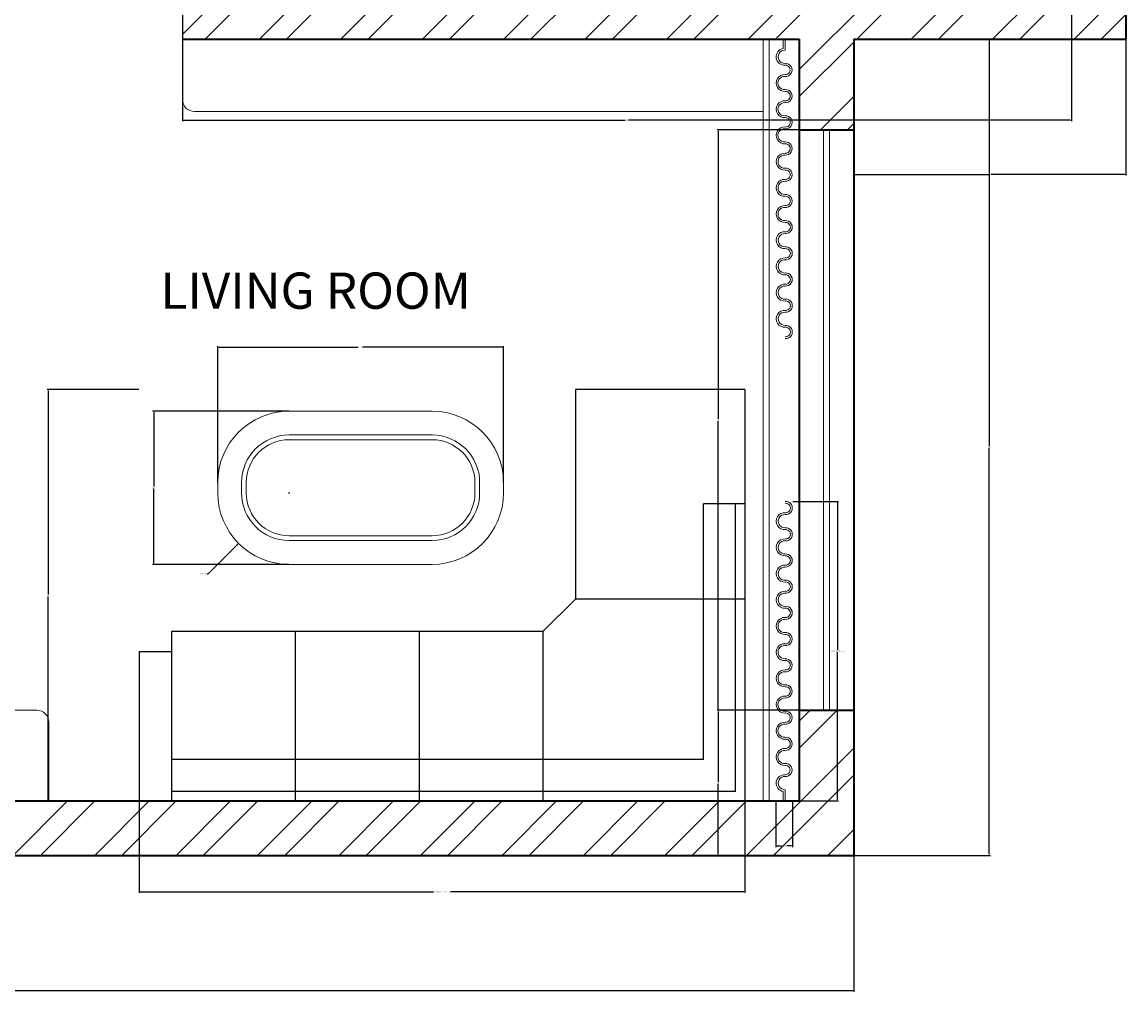
# Model space of a CAD drawing. Units: inches. Extents: x 3449 to 3843, y 1566 to 2054.
# Tile 4 of 8: x 3638 to 3820, y 1566 to 1726. Entities that reach past the tile are written whole.
import ezdxf

# ---------------------------------------------------------------- set-up
doc = ezdxf.new("R2010")
doc.units = ezdxf.units.IN
for name, color, linetype, lineweight in [('A-ANNO-DIMS', 2, 'Continuous', 18), ('A-AREA-IDEN', 7, 'Continuous', 25), ('A-FLOR-CASE', 7, 'Continuous', 20), ('A-FURN-DRAP', 32, 'Continuous', 13), ('A-GLAZ', 5, 'Continuous', 18), ('A-WALL', 7, 'Continuous', 35), ('A-WALL-PATT', 251, 'Continuous', 13), ('furn', 7, 'Continuous', 18)]:
    doc.layers.add(name, color=color, linetype=linetype, lineweight=lineweight)
doc.layers.add('B-FURNITURE', color=22, linetype='Continuous')
doc.styles.get("Standard").update_dxf_attribs({"font": 'arial.ttf'})
doc.dimstyles.get("Standard").update_dxf_attribs({"dimtxt": 0.18, "dimasz": 0.18, "dimexe": 0.18, "dimexo": 0.0625, "dimgap": 0.09, "dimtad": 0, "dimtih": 1, "dimtoh": 1, "dimdec": 4, "dimzin": 0, "dimdsep": 46, "dimtxsty": 'Standard', "dimcen": 0.09, "dimadec": 0, "dimazin": 0, "dimtfac": 1, "dimtdec": 4, "dimtofl": 0, "dimtmove": 0, "dimatfit": 3, "dimfxl": 1, "dimtolj": 1, "dimtzin": 0, "dimarcsym": 0})

# ---------------------------------------------------------------- blocks, each defined once
blk = doc.blocks.new('A$C4399559B')
at = {"layer": 'B-FURNITURE', "ltscale": 100}
for points in [[(-0.712, 0), (0, 0)], [(-0.712, 0), (-0.712, -0.88)], [(0, 0), (0, -0.88)], [(-0.712, -0.48), (-0.5377, -0.48)], [(-0.672, -1.688), (-0.672, -0.48)], [(-0.5377, -1.5537), (-0.5377, -0.48)], [(-0.712, -0.856), (-0.712, -1.728)], [(-0.712, -0.88), (-0.5377, -0.88)], [(-0.5377, -0.88), (0, -0.88)], [(0, -0.856), (0, -0.88)], [(0, -0.88), (0.136, -1.016)], [(0.136, -1.016), (1.696, -1.016)], [(0.136, -1.016), (0.136, -1.728)], [(0.656, -1.016), (0.656, -1.728)], [(1.176, -1.016), (1.176, -1.728)], [(1.696, -1.016), (1.696, -1.728)], [(1.696, -1.1016), (1.832, -1.1016)], [(1.832, -1.1016), (1.832, -1.728)], [(-0.5377, -1.5537), (1.696, -1.5537)], [(-0.672, -1.688), (1.696, -1.688)], [(-0.712, -1.728), (1.832, -1.728)]]:
    blk.add_lwpolyline(points, dxfattribs=at)
blk = doc.blocks.new('DRAPERY-PANEL')
for p, q in [((1.19, 47.95), (1.19, 49.52)), ((1.5, 47.66), (1.5, 49.52))]:
    blk.add_line(p, q)
for centre, radius, start, end in [((1.42, 46.57), 1.4, 99.481, 274.2422), ((1.42, 46.57), 1.09, 85.7578, 274.2422), ((1.55, 44.41), 1.09, 265.7578, 94.2422), ((1.55, 44.41), 0.776, 265.7578, 94.2422), ((1.4, 42.24), 1.4, 85.7578, 274.2422), ((1.4, 42.24), 1.09, 85.7578, 274.2422), ((1.56, 40.07), 1.09, 265.7578, 94.2422), ((1.56, 40.07), 0.776, 265.7578, 94.2422), ((1.4, 37.91), 1.4, 85.7578, 274.2422), ((1.4, 37.91), 1.09, 85.7578, 274.2422), ((1.56, 35.74), 1.09, 265.7578, 94.2422), ((1.56, 35.74), 0.776, 265.7578, 94.2422), ((1.4, 33.58), 1.4, 85.7578, 274.2422), ((1.4, 33.58), 1.09, 85.7578, 274.2422), ((1.56, 31.41), 1.09, 265.7578, 94.2422), ((1.56, 31.41), 0.776, 265.7578, 94.2422), ((1.41, 29.24), 1.4, 85.7578, 274.2422), ((1.41, 29.24), 1.09, 85.7578, 274.2422), ((1.57, 27.08), 1.09, 265.7578, 94.2422), ((1.57, 27.08), 0.776, 265.7578, 94.2422), ((1.41, 24.91), 1.4, 85.7578, 274.2422), ((1.41, 24.91), 1.09, 85.7578, 274.2422), ((1.57, 22.74), 1.09, 265.7578, 94.2422), ((1.41, 20.58), 1.4, 85.7578, 274.2422), ((1.57, 22.74), 0.776, 265.7578, 94.2422), ((1.41, 20.58), 1.09, 85.7578, 274.2422), ((1.58, 18.41), 1.09, 265.7578, 94.2422), ((1.58, 18.41), 0.776, 265.7578, 94.2422), ((1.42, 16.25), 1.4, 85.7578, 274.2422), ((1.42, 16.25), 1.09, 85.7578, 274.2422), ((1.58, 14.08), 1.09, 265.7578, 94.2422), ((1.58, 14.08), 0.776, 265.7578, 94.2422), ((1.42, 11.91), 1.4, 85.7578, 274.2422), ((1.42, 11.91), 1.09, 85.7578, 274.2422), ((1.58, 9.75), 1.09, 265.7578, 94.2422), ((1.58, 9.75), 0.776, 265.7578, 94.2422), ((1.43, 7.58), 1.4, 85.7578, 274.2422), ((1.43, 7.58), 1.09, 85.7578, 274.2422), ((1.59, 5.42), 1.09, 265.7578, 94.2422), ((1.59, 5.42), 0.776, 265.7578, 94.2422), ((1.43, 3.25), 1.4, 85.7578, 274.2422), ((1.43, 3.25), 1.09, 85.7578, 274.2422), ((1.59, 1.08), 1.09, 265.7578, 94.2422), ((1.59, 1.08), 0.776, 265.7578, 94.2422)]:
    blk.add_arc(centre, radius, start, end)
blk = doc.blocks.new('DRAPERY-PANEL-CAPPED')
for p, q in [((1.5, 1.86), (1.5, 0)), ((1.19, 1.57), (1.19, 0)), ((1.19, 0), (1.5, 0))]:
    blk.add_line(p, q)
for centre, radius, start, end in [((1.59, 48.44), 1.09, 265.7578, 94.2422), ((1.43, 46.27), 1.4, 85.7578, 274.2422), ((1.59, 48.44), 0.776, 265.7578, 94.2422), ((1.43, 46.27), 1.09, 85.7578, 274.2422), ((1.59, 44.1), 1.09, 265.7578, 94.2422), ((1.59, 44.1), 0.776, 265.7578, 94.2422), ((1.43, 41.94), 1.4, 85.7578, 274.2422), ((1.43, 41.94), 1.09, 85.7578, 274.2422), ((1.58, 39.77), 1.09, 265.7578, 94.2422), ((1.58, 39.77), 0.776, 265.7578, 94.2422), ((1.42, 37.6), 1.4, 85.7578, 274.2422), ((1.42, 37.6), 1.09, 85.7578, 274.2422), ((1.58, 35.44), 1.09, 265.7578, 94.2422), ((1.58, 35.44), 0.776, 265.7578, 94.2422), ((1.42, 33.27), 1.4, 85.7578, 274.2422), ((1.42, 33.27), 1.09, 85.7578, 274.2422), ((1.58, 31.11), 1.09, 265.7578, 94.2422), ((1.58, 31.11), 0.776, 265.7578, 94.2422), ((1.41, 28.94), 1.4, 85.7578, 274.2422), ((1.41, 28.94), 1.09, 85.7578, 274.2422), ((1.57, 26.77), 1.09, 265.7578, 94.2422), ((1.57, 26.77), 0.776, 265.7578, 94.2422), ((1.41, 24.61), 1.4, 85.7578, 274.2422), ((1.41, 24.61), 1.09, 85.7578, 274.2422), ((1.57, 22.44), 1.09, 265.7578, 94.2422), ((1.57, 22.44), 0.776, 265.7578, 94.2422), ((1.41, 20.28), 1.4, 85.7578, 274.2422), ((1.41, 20.28), 1.09, 85.7578, 274.2422), ((1.56, 18.11), 1.09, 265.7578, 94.2422), ((1.56, 18.11), 0.776, 265.7578, 94.2422), ((1.4, 15.94), 1.4, 85.7578, 274.2422), ((1.4, 15.94), 1.09, 85.7578, 274.2422), ((1.56, 13.78), 1.09, 265.7578, 94.2422), ((1.4, 11.61), 1.4, 85.7578, 274.2422), ((1.56, 13.78), 0.776, 265.7578, 94.2422), ((1.4, 11.61), 1.09, 85.7578, 274.2422), ((1.56, 9.45), 1.09, 265.7578, 94.2422), ((1.56, 9.45), 0.776, 265.7578, 94.2422), ((1.4, 7.28), 1.4, 85.7578, 274.2422), ((1.4, 7.28), 1.09, 85.7578, 274.2422), ((1.55, 5.11), 1.09, 265.7578, 94.2422), ((1.55, 5.11), 0.776, 265.7578, 94.2422), ((1.42, 2.95), 1.4, 85.7578, 260.519), ((1.42, 2.95), 1.09, 85.7578, 274.2422)]:
    blk.add_arc(centre, radius, start, end)
blk = doc.blocks.new('*D54')
at = {"layer": 'A-ANNO-DIMS', "color": 0, "lineweight": -2, "transparency": 16777216}
for p, q in [((3765.04, 1647.16), (3772.59, 1647.16)), ((3772.41, 1646.98), (3772.41, 1622.57)), ((3772.41, 1597.79), (3772.41, 1622.21)), ((3765.04, 1597.61), (3772.59, 1597.61))]:
    blk.add_line(p, q, dxfattribs=at)
at = {"layer": 'A-ANNO-DIMS', "color": 0, "transparency": 16777216}
for points in [[(3772.38, 1646.98), (3772.44, 1646.98), (3772.41, 1647.16)], [(3772.38, 1597.79), (3772.44, 1597.79), (3772.41, 1597.61)]]:
    blk.add_solid(points, dxfattribs=at)
at = {"layer": 'Defpoints', "color": 0, "transparency": 16777216}
for p in [(3764.98, 1647.16), (3772.41, 1647.16), (3764.98, 1597.61)]:
    blk.add_point(p, dxfattribs=at)
at = {"layer": 'A-ANNO-DIMS', "color": 0, "transparency": 16777216, "insert": (3772.41, 1622.39), "char_height": 0.18, "attachment_point": 5}
blk.add_mtext('\\A1;CAPPED DRAPE 50 TYP.', dxfattribs=at)
blk = doc.blocks.new('*D55')
at = {"layer": 'A-ANNO-DIMS', "color": 0, "lineweight": -2, "transparency": 16777216}
for p, q in [((3762.18, 1597.55), (3762.18, 1590)), ((3764.98, 1597.55), (3764.98, 1590)), ((3762.36, 1590.18), (3763.12, 1590.18)), ((3764.8, 1590.18), (3764.04, 1590.18))]:
    blk.add_line(p, q, dxfattribs=at)
at = {"layer": 'A-ANNO-DIMS', "color": 0, "transparency": 16777216}
for points in [[(3762.36, 1590.21), (3762.36, 1590.15), (3762.18, 1590.18)], [(3764.8, 1590.21), (3764.8, 1590.15), (3764.98, 1590.18)]]:
    blk.add_solid(points, dxfattribs=at)
at = {"layer": 'Defpoints', "color": 0, "transparency": 16777216}
for p in [(3762.18, 1597.61), (3764.98, 1597.61), (3764.98, 1590.18)]:
    blk.add_point(p, dxfattribs=at)
at = {"layer": 'A-ANNO-DIMS', "color": 0, "transparency": 16777216, "insert": (3763.58, 1590.18), "char_height": 0.18, "attachment_point": 5}
blk.add_mtext('\\A1;3 TYP.', dxfattribs=at)
blk = doc.blocks.new('*D62')
at = {"layer": 'A-ANNO-DIMS', "color": 0, "lineweight": -2, "transparency": 16777216}
for p, q in [((3656.93, 1597.55), (3656.93, 1582.41)), ((3757.09, 1597.55), (3757.09, 1582.41)), ((3657.11, 1582.59), (3705.6, 1582.59)), ((3756.91, 1582.59), (3708.42, 1582.59))]:
    blk.add_line(p, q, dxfattribs=at)
at = {"layer": 'A-ANNO-DIMS', "color": 0, "transparency": 16777216}
for points in [[(3657.11, 1582.62), (3657.11, 1582.56), (3656.93, 1582.59)], [(3756.91, 1582.62), (3756.91, 1582.56), (3757.09, 1582.59)]]:
    blk.add_solid(points, dxfattribs=at)
at = {"layer": 'Defpoints', "color": 0, "transparency": 16777216}
for p in [(3656.93, 1597.61), (3757.09, 1597.61), (3656.93, 1582.59)]:
    blk.add_point(p, dxfattribs=at)
at = {"layer": 'A-ANNO-DIMS', "color": 0, "transparency": 16777216, "insert": (3707.01, 1582.59), "char_height": 0.18, "attachment_point": 5}
blk.add_mtext('\\A1;SECTIONAL SOFA 100', dxfattribs=at)
blk = doc.blocks.new('*D63')
at = {"layer": 'A-ANNO-DIMS', "color": 0, "lineweight": -2, "transparency": 16777216}
for p, q in [((3656.87, 1665.65), (3641.73, 1665.65)), ((3641.91, 1665.47), (3641.91, 1631.81)), ((3641.91, 1597.79), (3641.91, 1631.45)), ((3656.87, 1597.61), (3641.73, 1597.61))]:
    blk.add_line(p, q, dxfattribs=at)
at = {"layer": 'A-ANNO-DIMS', "color": 0, "transparency": 16777216}
for points in [[(3641.88, 1665.47), (3641.94, 1665.47), (3641.91, 1665.65)], [(3641.88, 1597.79), (3641.94, 1597.79), (3641.91, 1597.61)]]:
    blk.add_solid(points, dxfattribs=at)
at = {"layer": 'Defpoints', "color": 0, "transparency": 16777216}
for p in [(3641.91, 1665.65), (3656.93, 1665.65), (3656.93, 1597.61)]:
    blk.add_point(p, dxfattribs=at)
at = {"layer": 'A-ANNO-DIMS', "color": 0, "transparency": 16777216, "insert": (3641.91, 1631.63), "char_height": 0.18, "attachment_point": 5}
blk.add_mtext('\\A1;68', dxfattribs=at)
blk = doc.blocks.new('*D91')
at = {"layer": 'A-ANNO-DIMS', "color": 0, "lineweight": -2, "transparency": 16777216}
for p, q in [((3664.09, 1732.55), (3664.09, 1710.03)), ((3811.09, 1732.55), (3811.09, 1710.03)), ((3664.27, 1710.21), (3737.31, 1710.21)), ((3810.91, 1710.21), (3737.87, 1710.21))]:
    blk.add_line(p, q, dxfattribs=at)
at = {"layer": 'A-ANNO-DIMS', "color": 0, "transparency": 16777216}
for points in [[(3664.27, 1710.24), (3664.27, 1710.18), (3664.09, 1710.21)], [(3810.91, 1710.24), (3810.91, 1710.18), (3811.09, 1710.21)]]:
    blk.add_solid(points, dxfattribs=at)
at = {"layer": 'Defpoints', "color": 0, "transparency": 16777216}
for p in [(3664.09, 1732.61), (3811.09, 1732.61), (3664.09, 1710.21)]:
    blk.add_point(p, dxfattribs=at)
at = {"layer": 'A-ANNO-DIMS', "color": 0, "transparency": 16777216, "insert": (3737.59, 1710.21), "char_height": 0.18, "attachment_point": 5}
blk.add_mtext('\\A1;147', dxfattribs=at)
blk = doc.blocks.new('*D99')
at = {"layer": 'A-ANNO-DIMS', "color": 0, "lineweight": -2, "transparency": 16777216}
for p, q in [((3481.09, 1588.55), (3481.09, 1566.03)), ((3775.09, 1588.55), (3775.09, 1566.03)), ((3481.27, 1566.21), (3627.8, 1566.21)), ((3774.91, 1566.21), (3628.38, 1566.21))]:
    blk.add_line(p, q, dxfattribs=at)
at = {"layer": 'A-ANNO-DIMS', "color": 0, "transparency": 16777216}
for points in [[(3481.27, 1566.24), (3481.27, 1566.18), (3481.09, 1566.21)], [(3774.91, 1566.24), (3774.91, 1566.18), (3775.09, 1566.21)]]:
    blk.add_solid(points, dxfattribs=at)
at = {"layer": 'Defpoints', "color": 0, "transparency": 16777216}
for p in [(3481.09, 1588.61), (3775.09, 1588.61), (3481.09, 1566.21)]:
    blk.add_point(p, dxfattribs=at)
at = {"layer": 'A-ANNO-DIMS', "color": 0, "transparency": 16777216, "insert": (3628.09, 1566.21), "char_height": 0.18, "attachment_point": 5}
blk.add_mtext('\\A1;294', dxfattribs=at)
blk = doc.blocks.new('*D100')
at = {"layer": 'A-ANNO-DIMS', "color": 0, "lineweight": -2, "transparency": 16777216}
for p, q in [((3775.15, 1723.61), (3797.67, 1723.61)), ((3797.49, 1723.43), (3797.49, 1656.3)), ((3797.49, 1588.79), (3797.49, 1655.93)), ((3775.15, 1588.61), (3797.67, 1588.61))]:
    blk.add_line(p, q, dxfattribs=at)
at = {"layer": 'A-ANNO-DIMS', "color": 0, "transparency": 16777216}
for points in [[(3797.46, 1723.43), (3797.52, 1723.43), (3797.49, 1723.61)], [(3797.46, 1588.79), (3797.52, 1588.79), (3797.49, 1588.61)]]:
    blk.add_solid(points, dxfattribs=at)
at = {"layer": 'Defpoints', "color": 0, "transparency": 16777216}
for p in [(3775.09, 1723.61), (3775.09, 1588.61), (3797.49, 1588.61)]:
    blk.add_point(p, dxfattribs=at)
at = {"layer": 'A-ANNO-DIMS', "color": 0, "transparency": 16777216, "insert": (3797.49, 1656.11), "char_height": 0.18, "attachment_point": 5}
blk.add_mtext('\\A1;135', dxfattribs=at)
blk = doc.blocks.new('*D101')
at = {"layer": 'A-ANNO-DIMS', "color": 0, "lineweight": -2, "transparency": 16777216}
for p, q in [((3775.03, 1708.61), (3752.51, 1708.61)), ((3752.69, 1708.43), (3752.69, 1660.8)), ((3752.69, 1612.79), (3752.69, 1660.43)), ((3775.03, 1612.61), (3752.51, 1612.61))]:
    blk.add_line(p, q, dxfattribs=at)
at = {"layer": 'A-ANNO-DIMS', "color": 0, "transparency": 16777216}
for points in [[(3752.66, 1708.43), (3752.72, 1708.43), (3752.69, 1708.61)], [(3752.66, 1612.79), (3752.72, 1612.79), (3752.69, 1612.61)]]:
    blk.add_solid(points, dxfattribs=at)
at = {"layer": 'Defpoints', "color": 0, "transparency": 16777216}
for p in [(3752.69, 1708.61), (3775.09, 1708.61), (3775.09, 1612.61)]:
    blk.add_point(p, dxfattribs=at)
at = {"layer": 'A-ANNO-DIMS', "color": 0, "transparency": 16777216, "insert": (3752.69, 1660.61), "char_height": 0.18, "attachment_point": 5}
blk.add_mtext('\\A1;96', dxfattribs=at)
blk = doc.blocks.new('*D102')
at = {"layer": 'A-ANNO-DIMS', "color": 0, "lineweight": -2, "transparency": 16777216}
for p, q in [((3775.09, 1723.55), (3775.09, 1701.03)), ((3820.09, 1723.55), (3820.09, 1701.03)), ((3775.27, 1701.21), (3797.36, 1701.21)), ((3819.91, 1701.21), (3797.81, 1701.21))]:
    blk.add_line(p, q, dxfattribs=at)
at = {"layer": 'A-ANNO-DIMS', "color": 0, "transparency": 16777216}
for points in [[(3775.27, 1701.24), (3775.27, 1701.18), (3775.09, 1701.21)], [(3819.91, 1701.24), (3819.91, 1701.18), (3820.09, 1701.21)]]:
    blk.add_solid(points, dxfattribs=at)
at = {"layer": 'Defpoints', "color": 0, "transparency": 16777216}
for p in [(3775.09, 1723.61), (3820.09, 1723.61), (3775.09, 1701.21)]:
    blk.add_point(p, dxfattribs=at)
at = {"layer": 'A-ANNO-DIMS', "color": 0, "transparency": 16777216, "insert": (3797.59, 1701.21), "char_height": 0.18, "attachment_point": 5}
blk.add_mtext('\\A1;45', dxfattribs=at)
blk = doc.blocks.new('*D115')
at = {"layer": 'A-ANNO-DIMS', "color": 0, "lineweight": -2, "transparency": 16777216}
for p, q in [((3775.03, 1612.61), (3752.51, 1612.61)), ((3752.69, 1612.43), (3752.69, 1600.79)), ((3752.69, 1588.79), (3752.69, 1600.43)), ((3775.03, 1588.61), (3752.51, 1588.61))]:
    blk.add_line(p, q, dxfattribs=at)
at = {"layer": 'A-ANNO-DIMS', "color": 0, "transparency": 16777216}
for points in [[(3752.66, 1612.43), (3752.72, 1612.43), (3752.69, 1612.61)], [(3752.66, 1588.79), (3752.72, 1588.79), (3752.69, 1588.61)]]:
    blk.add_solid(points, dxfattribs=at)
at = {"layer": 'Defpoints', "color": 0, "transparency": 16777216}
for p in [(3752.69, 1612.61), (3775.09, 1612.61), (3775.09, 1588.61)]:
    blk.add_point(p, dxfattribs=at)
at = {"layer": 'A-ANNO-DIMS', "color": 0, "transparency": 16777216, "insert": (3752.69, 1600.61), "char_height": 0.18, "attachment_point": 5}
blk.add_mtext('\\A1;24', dxfattribs=at)
blk = doc.blocks.new('*D119')
at = {"layer": 'A-ANNO-DIMS', "color": 0, "lineweight": -2, "transparency": 16777216}
for p, q in [((3669.93, 1650.33), (3669.93, 1672.84)), ((3670.11, 1672.66), (3693.15, 1672.66)), ((3716.99, 1672.66), (3693.94, 1672.66)), ((3717.17, 1650.33), (3717.17, 1672.84))]:
    blk.add_line(p, q, dxfattribs=at)
at = {"layer": 'A-ANNO-DIMS', "color": 0, "transparency": 16777216}
for points in [[(3670.11, 1672.69), (3670.11, 1672.63), (3669.93, 1672.66)], [(3716.99, 1672.69), (3716.99, 1672.63), (3717.17, 1672.66)]]:
    blk.add_solid(points, dxfattribs=at)
at = {"layer": 'Defpoints', "color": 0, "transparency": 16777216}
for p in [(3717.17, 1672.66), (3669.93, 1650.26), (3717.17, 1650.26)]:
    blk.add_point(p, dxfattribs=at)
at = {"layer": 'A-ANNO-DIMS', "color": 0, "transparency": 16777216, "insert": (3693.55, 1672.66), "char_height": 0.18, "attachment_point": 5}
blk.add_mtext('\\A1;47.24', dxfattribs=at)
blk = doc.blocks.new('*D120')
at = {"layer": 'A-ANNO-DIMS', "color": 0, "lineweight": -2, "transparency": 16777216}
for p, q in [((3681.67, 1662.08), (3659.16, 1662.08)), ((3659.34, 1661.9), (3659.34, 1649.59)), ((3659.34, 1636.92), (3659.34, 1649.22)), ((3681.67, 1636.74), (3659.16, 1636.74))]:
    blk.add_line(p, q, dxfattribs=at)
at = {"layer": 'A-ANNO-DIMS', "color": 0, "transparency": 16777216}
for points in [[(3659.31, 1661.9), (3659.37, 1661.9), (3659.34, 1662.08)], [(3659.31, 1636.92), (3659.37, 1636.92), (3659.34, 1636.74)]]:
    blk.add_solid(points, dxfattribs=at)
at = {"layer": 'Defpoints', "color": 0, "transparency": 16777216}
for p in [(3659.34, 1662.08), (3681.74, 1662.08), (3681.74, 1636.74)]:
    blk.add_point(p, dxfattribs=at)
at = {"layer": 'A-ANNO-DIMS', "color": 0, "transparency": 16777216, "insert": (3659.34, 1649.41), "char_height": 0.18, "attachment_point": 5}
blk.add_mtext('\\A1;25.34', dxfattribs=at)
blk = doc.blocks.new('*D125')
at = {"layer": 'A-ANNO-DIMS', "color": 0, "lineweight": -2, "transparency": 16777216}
for p, q in [((3681.65, 1648.55), (3681.83, 1648.55)), ((3681.74, 1648.46), (3681.74, 1648.64)), ((3668.37, 1635.18), (3673.26, 1640.07)), ((3668.19, 1635.18), (3668.37, 1635.18))]:
    blk.add_line(p, q, dxfattribs=at)
at = {"layer": 'A-ANNO-DIMS', "color": 0, "transparency": 16777216}
blk.add_solid([(3673.24, 1640.09), (3673.28, 1640.05), (3673.39, 1640.2)], dxfattribs=at)
at = {"layer": 'Defpoints', "color": 0, "transparency": 16777216}
for p in [(3681.74, 1648.55), (3673.39, 1640.2)]:
    blk.add_point(p, dxfattribs=at)
at = {"layer": 'A-ANNO-DIMS', "color": 0, "transparency": 16777216, "insert": (3667.53, 1635.18), "char_height": 0.18, "attachment_point": 5}
blk.add_mtext('\\A1;4X R11.81', dxfattribs=at)

msp = doc.modelspace()

# ---------------------------------------------------------------- hatches: boundary and pattern name
at = {"layer": 'A-WALL-PATT'}
h = msp.add_hatch(dxfattribs=at)
h.set_pattern_fill('ANSI32', color=256)
edge = h.paths.add_edge_path()
edge.add_line((3481.088, 2022.6144), (3508.088, 2022.6144))
edge.add_line((3508.088, 2022.6144), (3508.088, 2031.6144))
edge.add_line((3508.088, 2031.6144), (3472.088, 2031.6144))
edge.add_line((3472.088, 2031.6144), (3472.088, 1779.6144))
edge.add_line((3472.088, 1779.6144), (3481.088, 1779.6144))
edge.add_line((3481.088, 1779.6144), (3481.088, 1839.6144))
edge.add_line((3481.088, 1839.6144), (3571.088, 1839.6144))
edge.add_line((3571.088, 1839.6144), (3571.088, 1824.3194))
edge.add_line((3571.088, 1824.3194), (3571.088, 1821.6144))
edge.add_line((3571.088, 1821.6144), (3580.088, 1821.6144))
edge.add_line((3580.088, 1821.6144), (3580.088, 1825.1908))
edge.add_ellipse((3580.1411, 1825.2442), major_axis=(0, 0.0754), ratio=0.99913951, start_angle=90, end_angle=135.183195, ccw=False)
edge.add_line((3580.0017, 1825.3196), (3580.0658, 1825.3196))
edge.add_line((3580.0658, 1825.3196), (3580.066, 1839.6365))
edge.add_line((3580.066, 1839.6365), (3616.088, 1839.6365))
edge.add_line((3616.088, 1839.6365), (3616.088, 1848.6144))
edge.add_line((3616.088, 1848.6144), (3610.088, 1848.6144))
edge.add_line((3610.088, 1848.6144), (3574.088, 1848.6144))
edge.add_line((3574.088, 1848.6144), (3481.088, 1848.6144))
edge.add_line((3481.088, 1848.6144), (3481.088, 1872.6144))
edge.add_line((3481.088, 1872.6144), (3481.088, 2022.6144))
h.paths.add_polyline_path([(3550.088, 1779.6144), (3616.088, 1779.6144), (3616.088, 1791.6144), (3505.088, 1791.6144), (3505.088, 1779.6144), (3541.088, 1779.6144), (3541.088, 1657.6144), (3481.088, 1657.6144), (3481.088, 1588.6144), (3496.088, 1588.6144), (3496.088, 1594.6144), (3496.088, 1597.6144), (3490.088, 1597.6144), (3490.088, 1648.6144), (3550.088, 1648.6144)])
h.paths.add_polyline_path([(3775.088, 1612.6144), (3766.088, 1612.6144), (3766.088, 1597.6144), (3536.088, 1597.6144), (3536.088, 1588.6144), (3775.088, 1588.6144)])
h.paths.add_polyline_path([(3820.088, 1756.6144), (3811.088, 1756.6144), (3811.088, 1732.6144), (3664.088, 1732.6144), (3664.088, 1723.6144), (3766.088, 1723.6144), (3766.088, 1708.6144), (3775.088, 1708.6144), (3775.088, 1723.6144), (3820.088, 1723.6144)])
h.paths.add_polyline_path([(3820.088, 1986.6144), (3745.088, 1986.6144), (3745.088, 2010.6144), (3664.088, 2010.6144), (3664.088, 1992.6144), (3652.088, 1992.6144), (3652.088, 1983.6144), (3664.088, 1983.6144), (3664.088, 1893.6144), (3648.793, 1893.6144), (3607.088, 1893.6144), (3607.088, 1884.6144), (3673.088, 1884.6144), (3673.088, 2001.6144), (3736.088, 2001.6144), (3736.088, 1977.6144), (3811.088, 1977.6144), (3811.088, 1949.1144), (3820.088, 1949.1144)])
h.paths.add_polyline_path([(3628.088, 1992.6144), (3616.088, 1992.6144), (3616.088, 2031.6144), (3580.088, 2031.6144), (3580.088, 2022.6144), (3607.088, 2022.6144), (3607.088, 1921.6144), (3613.088, 1921.6144), (3616.088, 1921.6144), (3616.088, 1983.6144), (3628.088, 1983.6144)])
h.paths.add_polyline_path([(3820.088, 1877.1144), (3811.088, 1877.1144), (3811.088, 1848.6144), (3664.088, 1848.6144), (3664.088, 1839.6144), (3700.088, 1839.6144), (3811.088, 1839.6144), (3811.088, 1815.6144), (3820.088, 1815.6144)])

# ---------------------------------------------------------------- linework, layer by layer
at = {"layer": 'A-FLOR-CASE'}
for p, q in [((3664.088, 1770.6144), (3664.088, 1713.6144)), ((3666.088, 1711.6144), (3760.088, 1711.6144))]:
    msp.add_line(p, q, dxfattribs=at)
msp.add_arc((3666.088, 1713.6144), 2, 180, 270, dxfattribs=at)
at = {"layer": 'A-FURN-DRAP'}
for p, q in [((3760.088, 1723.6144), (3760.088, 1597.6144)), ((3761.088, 1723.6144), (3761.088, 1597.6144))]:
    msp.add_line(p, q, dxfattribs=at)
at = {"layer": 'A-GLAZ'}
for p, q in [((3770.088, 1708.6144), (3770.088, 1612.6144)), ((3771.088, 1708.6144), (3771.088, 1612.6144))]:
    msp.add_line(p, q, dxfattribs=at)
at = {"layer": 'A-WALL'}
for p, q in [((3820.088, 1756.6144), (3820.088, 1723.6144)), ((3664.088, 1723.6144), (3766.088, 1723.6144)), ((3766.088, 1723.6144), (3766.088, 1597.6144)), ((3775.088, 1723.6144), (3775.088, 1612.6144)), ((3775.088, 1723.6144), (3820.088, 1723.6144)), ((3766.088, 1708.6144), (3775.088, 1708.6144)), ((3766.088, 1612.6144), (3775.088, 1612.6144)), ((3775.088, 1612.6144), (3775.088, 1588.6144)), ((3536.088, 1597.6144), (3766.088, 1597.6144)), ((3536.088, 1588.6144), (3775.088, 1588.6144))]:
    msp.add_line(p, q, dxfattribs=at)
at = {"layer": 'furn'}
for points in [[(3705.3588, 1636.7359), (3681.7368, 1636.7359, -0.41421356), (3669.9258, 1648.5469), (3669.9258, 1650.2649, -0.41421356), (3681.7368, 1662.0759), (3705.3588, 1662.0759, -0.41421356), (3717.1699, 1650.2649), (3717.1699, 1648.5469, -0.41421356)], [(3705.3588, 1640.6729), (3681.7368, 1640.6729, -0.41421356), (3673.8628, 1648.5469), (3673.8628, 1650.2649, -0.41421356), (3681.7368, 1658.1389), (3705.3588, 1658.1389, -0.41421356), (3713.2329, 1650.2649), (3713.2329, 1648.5469, -0.41421356)], [(3705.3588, 1641.4603), (3681.7368, 1641.4603, -0.41421356), (3674.6502, 1648.5469), (3674.6502, 1650.2649, -0.41421356), (3681.7368, 1657.3515), (3705.3588, 1657.3515, -0.41421356), (3712.4455, 1650.2649), (3712.4455, 1648.5469, -0.41421356)], [(3609.0062, 1597.6144), (3642.0062, 1597.6144), (3642.0062, 1610.6144, 0.41421356), (3640.0062, 1612.6144), (3611.0062, 1612.6144, 0.41421356), (3609.0062, 1610.6144)]]:
    msp.add_lwpolyline(points, format="xyb", close=True, dxfattribs=at)

# ---------------------------------------------------------------- block references
at = {"layer": 'A-FURN-DRAP'}
for name, p in [('DRAPERY-PANEL', (3762.247, 1674.096)), ('DRAPERY-PANEL-CAPPED', (3762.247, 1597.614))]:
    msp.add_blockref(name, p, dxfattribs=at)
at = {"layer": 'furn', "xscale": -39.3701, "yscale": 39.3701, "zscale": 39.3701}
msp.add_blockref('A$C4399559B', (3729.0557, 1665.6461), dxfattribs=at)

# ---------------------------------------------------------------- texts
at = {"layer": 'A-AREA-IDEN', "insert": (3660.4473, 1685.0007), "char_height": 6, "attachment_point": 1}
msp.add_mtext_dynamic_manual_height_columns('LIVING ROOM', width=95.638287, gutter_width=12.5, heights=[0], dxfattribs=at)

# ---------------------------------------------------------------- dimensions: what is measured, and where the dimension line sits
at = {"layer": 'A-ANNO-DIMS'}
for base, p1, p2, angle, override, picture, middle in [((3664.088, 1710.2144), (3811.088, 1732.6144), (3664.088, 1732.6144), 180, {"dimdec": 0, "dimlfac": 1, "dimrnd": 0, "dimzin": 0, "dimdsep": 46, "dimlunit": 2}, '*D91', (3737.588, 1710.2144)), ((3797.488, 1588.6144), (3775.088, 1723.6144), (3775.088, 1588.6144), 270, {"dimdec": 0, "dimlfac": 1, "dimrnd": 0, "dimzin": 0, "dimdsep": 46, "dimlunit": 2}, '*D100', (3797.488, 1656.1144)), ((3775.088, 1701.2144), (3820.088, 1723.6144), (3775.088, 1723.6144), 180, {"dimdec": 0, "dimlfac": 1, "dimrnd": 0, "dimzin": 0, "dimdsep": 46, "dimlunit": 2}, '*D102', (3797.588, 1701.2144)), ((3752.688, 1708.6144), (3775.088, 1612.6144), (3775.088, 1708.6144), 90, {"dimdec": 0, "dimlfac": 1, "dimrnd": 0, "dimzin": 0, "dimdsep": 46, "dimlunit": 2}, '*D101', (3752.688, 1660.6144)), ((3641.9061, 1665.6461), (3656.9297, 1597.6144), (3656.9297, 1665.6461), 90, {"dimdec": 0, "dimlfac": 1, "dimrnd": 0, "dimzin": 0, "dimdsep": 46, "dimlunit": 2}, '*D63', (3641.9061, 1631.6302)), ((3659.3368, 1662.0759), (3681.7368, 1636.7359), (3681.7368, 1662.0759), 90, {"dimdec": 2, "dimlfac": 1, "dimrnd": 0, "dimzin": 0, "dimdsep": 46, "dimlunit": 2}, '*D120', (3659.3368, 1649.4059)), ((3752.688, 1612.6144), (3775.088, 1588.6144), (3775.088, 1612.6144), 90, {"dimdec": 0, "dimlfac": 1, "dimrnd": 0, "dimzin": 0, "dimdsep": 46, "dimlunit": 2}, '*D115', (3752.688, 1600.6144)), ((3481.088, 1566.2144), (3775.088, 1588.6144), (3481.088, 1588.6144), 180, {"dimdec": 0, "dimlfac": 1, "dimrnd": 0, "dimzin": 0, "dimdsep": 46, "dimlunit": 2}, '*D99', (3628.088, 1566.2144))]:
    dim = msp.add_linear_dim(base=base, p1=p1, p2=p2, angle=angle, dimstyle='Standard', override=override, dxfattribs=at)
    dim.commit()
    dim.dimension.update_dxf_attribs({"geometry": picture, "text_midpoint": middle})
dim = msp.add_linear_dim(base=(3717.1699, 1672.6649), p1=(3669.9258, 1650.2649), p2=(3717.1699, 1650.2649), dimstyle='Standard', override={"dimdec": 2, "dimlfac": 1, "dimrnd": 0, "dimzin": 0, "dimdsep": 46, "dimlunit": 2}, dxfattribs=at)
dim.commit()
dim.dimension.update_dxf_attribs({"geometry": '*D119', "text_midpoint": (3693.5478, 1672.6649)})
dim = msp.add_radius_dim(center=(3681.7368, 1648.5469), mpoint=(3673.3852, 1640.1952), text='4X <>', dimstyle='Standard', override={"dimdec": 2, "dimlfac": 1, "dimrnd": 0, "dimzin": 0, "dimdsep": 46, "dimlunit": 2}, dxfattribs=at)
dim.commit()
dim.dimension.update_dxf_attribs({"geometry": '*D125', "text_midpoint": (3667.5348, 1635.1842), "dimtype": 164})
for base, p1, p2, angle, text, picture, middle in [((3772.4086, 1647.1623), (3764.9764, 1597.6144), (3764.9764, 1647.1623), 90, 'CAPPED DRAPE <> TYP.', '*D54', (3772.4086, 1622.3883)), ((3656.9297, 1582.5908), (3757.0872, 1597.6144), (3656.9297, 1597.6144), 180, 'SECTIONAL SOFA <>', '*D62', (3707.0085, 1582.5908))]:
    dim = msp.add_linear_dim(base=base, p1=p1, p2=p2, angle=angle, text=text, dimstyle='Standard', override={"dimdec": 0, "dimlfac": 1, "dimrnd": 0, "dimzin": 0, "dimdsep": 46, "dimlunit": 2}, dxfattribs=at)
    dim.commit()
    dim.dimension.update_dxf_attribs({"geometry": picture, "text_midpoint": middle})
dim = msp.add_linear_dim(base=(3764.9764, 1590.1822), p1=(3762.1789, 1597.6144), p2=(3764.9764, 1597.6144), text='<> TYP.', dimstyle='Standard', override={"dimdec": 0, "dimlfac": 1, "dimrnd": 0, "dimzin": 0, "dimdsep": 46, "dimlunit": 2}, dxfattribs=at)
dim.commit()
dim.dimension.update_dxf_attribs({"geometry": '*D55', "text_midpoint": (3763.5777, 1590.1822)})

doc.saveas('drawing.dxf')
